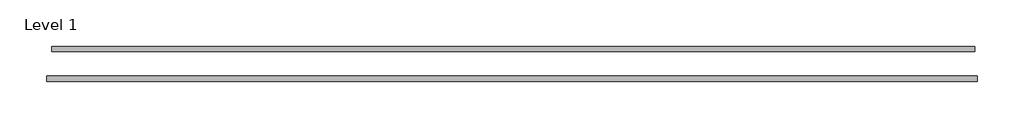
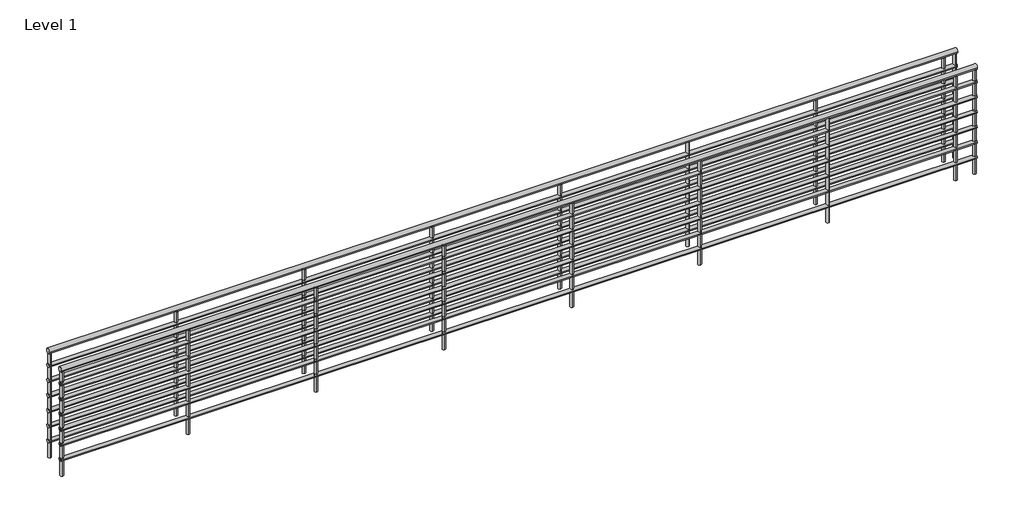
# One storey, part 2 of 2: 2 railings.
"""IFC4 building model written with IfcOpenShell, lengths in millimetres."""

from ifc_helpers import new_model, si_unit, point, frame, frame_2d, origin, origin_with_axes, place, context, project, spatial, circle_curve, trimmed, segment, composite_curve, outline, extrude, element, save

model = new_model("IFC4")

# Units and contexts
model_context = context("Model", 3, world=origin())
ifc_project = project(units=[si_unit("LENGTHUNIT", "METRE", prefix="MILLI")], contexts=[model_context])

# Site, building, storey
site = spatial("IfcSite", under=ifc_project)
building = spatial("IfcBuilding", under=site)
storey = spatial("IfcBuildingStorey", under=building, Name="Level 1", Elevation=0.0)

# Railings
placement = place(None, origin())
element("IfcRailing", 1, ObjectType="900mm Pipe", at=placement, inside=storey, context=model_context, shape_type="SweptSolid", body=[
    extrude(outline(composite_curve([segment(trimmed(circle_curve(frame_2d((34329.0024844, 880.0)), 20.0), [point((34309.0024844, 880.0))], [point((34349.0024844, 880.0))], False, "CARTESIAN"), True, "CONTINUOUS"), segment(trimmed(circle_curve(frame_2d((34329.0024844, 880.0)), 20.0), [point((34349.0024844, 880.0))], [point((34309.0024844, 880.0))], False, "CARTESIAN"), True, "CONTINUOUS")], self_intersect=False)), frame((-2703.3852997, 0.0, 0.0), z_axis=(1.0, 0.0, 0.0), x_axis=(0.0, 1.0, 0.0)), (0.0, 0.0, 1.0), 7100.0),
    extrude(outline(composite_curve([segment(trimmed(circle_curve(frame_2d((34329.0024844, 760.0)), 15.0), [point((34344.0024844, 760.0))], [point((34314.0024844, 760.0))], False, "CARTESIAN"), True, "CONTINUOUS"), segment(trimmed(circle_curve(frame_2d((34329.0024844, 760.0)), 15.0), [point((34314.0024844, 760.0))], [point((34344.0024844, 760.0))], False, "CARTESIAN"), True, "CONTINUOUS")], self_intersect=False)), frame((-2703.3852997, 0.0, 0.0), z_axis=(1.0, 0.0, 0.0), x_axis=(0.0, 1.0, 0.0)), (0.0, 0.0, 1.0), 7100.0),
    extrude(outline(composite_curve([segment(trimmed(circle_curve(frame_2d((34329.0024844, 635.0)), 15.0), [point((34344.0024844, 635.0))], [point((34314.0024844, 635.0))], False, "CARTESIAN"), True, "CONTINUOUS"), segment(trimmed(circle_curve(frame_2d((34329.0024844, 635.0)), 15.0), [point((34314.0024844, 635.0))], [point((34344.0024844, 635.0))], False, "CARTESIAN"), True, "CONTINUOUS")], self_intersect=False)), frame((-2703.3852997, 0.0, 0.0), z_axis=(1.0, 0.0, 0.0), x_axis=(0.0, 1.0, 0.0)), (0.0, 0.0, 1.0), 7100.0),
    extrude(outline(composite_curve([segment(trimmed(circle_curve(frame_2d((34329.0024844, 510.0)), 15.0), [point((34344.0024844, 510.0))], [point((34314.0024844, 510.0))], False, "CARTESIAN"), True, "CONTINUOUS"), segment(trimmed(circle_curve(frame_2d((34329.0024844, 510.0)), 15.0), [point((34314.0024844, 510.0))], [point((34344.0024844, 510.0))], False, "CARTESIAN"), True, "CONTINUOUS")], self_intersect=False)), frame((-2703.3852997, 0.0, 0.0), z_axis=(1.0, 0.0, 0.0), x_axis=(0.0, 1.0, 0.0)), (0.0, 0.0, 1.0), 7100.0),
    extrude(outline(composite_curve([segment(trimmed(circle_curve(frame_2d((34329.0024844, 385.0)), 15.0), [point((34344.0024844, 385.0))], [point((34314.0024844, 385.0))], False, "CARTESIAN"), True, "CONTINUOUS"), segment(trimmed(circle_curve(frame_2d((34329.0024844, 385.0)), 15.0), [point((34314.0024844, 385.0))], [point((34344.0024844, 385.0))], False, "CARTESIAN"), True, "CONTINUOUS")], self_intersect=False)), frame((-2703.3852997, 0.0, 0.0), z_axis=(1.0, 0.0, 0.0), x_axis=(0.0, 1.0, 0.0)), (0.0, 0.0, 1.0), 7100.0),
    extrude(outline(composite_curve([segment(trimmed(circle_curve(frame_2d((34329.0024844, 260.0)), 15.0), [point((34344.0024844, 260.0))], [point((34314.0024844, 260.0))], False, "CARTESIAN"), True, "CONTINUOUS"), segment(trimmed(circle_curve(frame_2d((34329.0024844, 260.0)), 15.0), [point((34314.0024844, 260.0))], [point((34344.0024844, 260.0))], False, "CARTESIAN"), True, "CONTINUOUS")], self_intersect=False)), frame((-2703.3852997, 0.0, 0.0), z_axis=(1.0, 0.0, 0.0), x_axis=(0.0, 1.0, 0.0)), (0.0, 0.0, 1.0), 7100.0),
    extrude(outline(composite_curve([segment(trimmed(circle_curve(frame_2d((34329.0024844, 135.0)), 15.0), [point((34344.0024844, 135.0))], [point((34314.0024844, 135.0))], False, "CARTESIAN"), True, "CONTINUOUS"), segment(trimmed(circle_curve(frame_2d((34329.0024844, 135.0)), 15.0), [point((34314.0024844, 135.0))], [point((34344.0024844, 135.0))], False, "CARTESIAN"), True, "CONTINUOUS")], self_intersect=False)), frame((-2703.3852997, 0.0, 0.0), z_axis=(1.0, 0.0, 0.0), x_axis=(0.0, 1.0, 0.0)), (0.0, 0.0, 1.0), 7100.0),
    extrude(outline(composite_curve([segment(trimmed(circle_curve(frame_2d((4296.6147003, 34329.0024844)), 12.5), [point((4296.6147003, 34341.5024844))], [point((4296.6147003, 34316.5024844))], False, "CARTESIAN"), True, "CONTINUOUS"), segment(trimmed(circle_curve(frame_2d((4296.6147003, 34329.0024844)), 12.5), [point((4296.6147003, 34316.5024844))], [point((4296.6147003, 34341.5024844))], False, "CARTESIAN"), True, "CONTINUOUS")], self_intersect=False)), origin_with_axes(), (0.0, 0.0, 1.0), 860.0),
    extrude(outline(composite_curve([segment(trimmed(circle_curve(frame_2d((3296.6147003, 34329.0024844)), 12.5), [point((3296.6147003, 34341.5024844))], [point((3296.6147003, 34316.5024844))], False, "CARTESIAN"), True, "CONTINUOUS"), segment(trimmed(circle_curve(frame_2d((3296.6147003, 34329.0024844)), 12.5), [point((3296.6147003, 34316.5024844))], [point((3296.6147003, 34341.5024844))], False, "CARTESIAN"), True, "CONTINUOUS")], self_intersect=False)), origin_with_axes(), (0.0, 0.0, 1.0), 860.0),
    extrude(outline(composite_curve([segment(trimmed(circle_curve(frame_2d((2296.6147003, 34329.0024844)), 12.5), [point((2296.6147003, 34341.5024844))], [point((2296.6147003, 34316.5024844))], False, "CARTESIAN"), True, "CONTINUOUS"), segment(trimmed(circle_curve(frame_2d((2296.6147003, 34329.0024844)), 12.5), [point((2296.6147003, 34316.5024844))], [point((2296.6147003, 34341.5024844))], False, "CARTESIAN"), True, "CONTINUOUS")], self_intersect=False)), origin_with_axes(), (0.0, 0.0, 1.0), 860.0),
    extrude(outline(composite_curve([segment(trimmed(circle_curve(frame_2d((1296.6147003, 34329.0024844)), 12.5), [point((1296.6147003, 34341.5024844))], [point((1296.6147003, 34316.5024844))], False, "CARTESIAN"), True, "CONTINUOUS"), segment(trimmed(circle_curve(frame_2d((1296.6147003, 34329.0024844)), 12.5), [point((1296.6147003, 34316.5024844))], [point((1296.6147003, 34341.5024844))], False, "CARTESIAN"), True, "CONTINUOUS")], self_intersect=False)), origin_with_axes(), (0.0, 0.0, 1.0), 860.0),
    extrude(outline(composite_curve([segment(trimmed(circle_curve(frame_2d((296.6147003, 34329.0024844)), 12.5), [point((296.6147003, 34341.5024844))], [point((296.6147003, 34316.5024844))], False, "CARTESIAN"), True, "CONTINUOUS"), segment(trimmed(circle_curve(frame_2d((296.6147003, 34329.0024844)), 12.5), [point((296.6147003, 34316.5024844))], [point((296.6147003, 34341.5024844))], False, "CARTESIAN"), True, "CONTINUOUS")], self_intersect=False)), origin_with_axes(), (0.0, 0.0, 1.0), 860.0),
    extrude(outline(composite_curve([segment(trimmed(circle_curve(frame_2d((-703.3852997, 34329.0024844)), 12.5), [point((-703.3852997, 34341.5024844))], [point((-703.3852997, 34316.5024844))], False, "CARTESIAN"), True, "CONTINUOUS"), segment(trimmed(circle_curve(frame_2d((-703.3852997, 34329.0024844)), 12.5), [point((-703.3852997, 34316.5024844))], [point((-703.3852997, 34341.5024844))], False, "CARTESIAN"), True, "CONTINUOUS")], self_intersect=False)), origin_with_axes(), (0.0, 0.0, 1.0), 860.0),
    extrude(outline(composite_curve([segment(trimmed(circle_curve(frame_2d((-1703.3852997, 34329.0024844)), 12.5), [point((-1703.3852997, 34341.5024844))], [point((-1703.3852997, 34316.5024844))], False, "CARTESIAN"), True, "CONTINUOUS"), segment(trimmed(circle_curve(frame_2d((-1703.3852997, 34329.0024844)), 12.5), [point((-1703.3852997, 34316.5024844))], [point((-1703.3852997, 34341.5024844))], False, "CARTESIAN"), True, "CONTINUOUS")], self_intersect=False)), origin_with_axes(), (0.0, 0.0, 1.0), 860.0),
    extrude(outline(composite_curve([segment(trimmed(circle_curve(frame_2d((4384.1147003, 34329.0024844)), 12.5), [point((4384.1147003, 34341.5024844))], [point((4384.1147003, 34316.5024844))], False, "CARTESIAN"), True, "CONTINUOUS"), segment(trimmed(circle_curve(frame_2d((4384.1147003, 34329.0024844)), 12.5), [point((4384.1147003, 34316.5024844))], [point((4384.1147003, 34341.5024844))], False, "CARTESIAN"), True, "CONTINUOUS")], self_intersect=False)), origin_with_axes(), (0.0, 0.0, 1.0), 860.0),
    extrude(outline(composite_curve([segment(trimmed(circle_curve(frame_2d((-2690.8852997, 34329.0024844)), 12.5), [point((-2690.8852997, 34341.5024844))], [point((-2690.8852997, 34316.5024844))], False, "CARTESIAN"), True, "CONTINUOUS"), segment(trimmed(circle_curve(frame_2d((-2690.8852997, 34329.0024844)), 12.5), [point((-2690.8852997, 34316.5024844))], [point((-2690.8852997, 34341.5024844))], False, "CARTESIAN"), True, "CONTINUOUS")], self_intersect=False)), origin_with_axes(), (0.0, 0.0, 1.0), 860.0),
])
element("IfcRailing", 2, ObjectType="900mm Pipe", at=placement, inside=storey, context=model_context, shape_type="SweptSolid", body=[
    extrude(outline(composite_curve([segment(trimmed(circle_curve(frame_2d((34099.2348375, 880.0)), 20.0), [point((34079.2348375, 880.0))], [point((34119.2348375, 880.0))], False, "CARTESIAN"), True, "CONTINUOUS"), segment(trimmed(circle_curve(frame_2d((34099.2348375, 880.0)), 20.0), [point((34119.2348375, 880.0))], [point((34079.2348375, 880.0))], False, "CARTESIAN"), True, "CONTINUOUS")], self_intersect=False)), frame((-2741.5918674, 0.0, 0.0), z_axis=(1.0, 0.0, 0.0), x_axis=(0.0, 1.0, 0.0)), (0.0, 0.0, 1.0), 7160.0),
    extrude(outline(composite_curve([segment(trimmed(circle_curve(frame_2d((34099.2348375, 760.0)), 15.0), [point((34114.2348375, 760.0))], [point((34084.2348375, 760.0))], False, "CARTESIAN"), True, "CONTINUOUS"), segment(trimmed(circle_curve(frame_2d((34099.2348375, 760.0)), 15.0), [point((34084.2348375, 760.0))], [point((34114.2348375, 760.0))], False, "CARTESIAN"), True, "CONTINUOUS")], self_intersect=False)), frame((-2741.5918674, 0.0, 0.0), z_axis=(1.0, 0.0, 0.0), x_axis=(0.0, 1.0, 0.0)), (0.0, 0.0, 1.0), 7160.0),
    extrude(outline(composite_curve([segment(trimmed(circle_curve(frame_2d((34099.2348375, 635.0)), 15.0), [point((34114.2348375, 635.0))], [point((34084.2348375, 635.0))], False, "CARTESIAN"), True, "CONTINUOUS"), segment(trimmed(circle_curve(frame_2d((34099.2348375, 635.0)), 15.0), [point((34084.2348375, 635.0))], [point((34114.2348375, 635.0))], False, "CARTESIAN"), True, "CONTINUOUS")], self_intersect=False)), frame((-2741.5918674, 0.0, 0.0), z_axis=(1.0, 0.0, 0.0), x_axis=(0.0, 1.0, 0.0)), (0.0, 0.0, 1.0), 7160.0),
    extrude(outline(composite_curve([segment(trimmed(circle_curve(frame_2d((34099.2348375, 510.0)), 15.0), [point((34114.2348375, 510.0))], [point((34084.2348375, 510.0))], False, "CARTESIAN"), True, "CONTINUOUS"), segment(trimmed(circle_curve(frame_2d((34099.2348375, 510.0)), 15.0), [point((34084.2348375, 510.0))], [point((34114.2348375, 510.0))], False, "CARTESIAN"), True, "CONTINUOUS")], self_intersect=False)), frame((-2741.5918674, 0.0, 0.0), z_axis=(1.0, 0.0, 0.0), x_axis=(0.0, 1.0, 0.0)), (0.0, 0.0, 1.0), 7160.0),
    extrude(outline(composite_curve([segment(trimmed(circle_curve(frame_2d((34099.2348375, 385.0)), 15.0), [point((34114.2348375, 385.0))], [point((34084.2348375, 385.0))], False, "CARTESIAN"), True, "CONTINUOUS"), segment(trimmed(circle_curve(frame_2d((34099.2348375, 385.0)), 15.0), [point((34084.2348375, 385.0))], [point((34114.2348375, 385.0))], False, "CARTESIAN"), True, "CONTINUOUS")], self_intersect=False)), frame((-2741.5918674, 0.0, 0.0), z_axis=(1.0, 0.0, 0.0), x_axis=(0.0, 1.0, 0.0)), (0.0, 0.0, 1.0), 7160.0),
    extrude(outline(composite_curve([segment(trimmed(circle_curve(frame_2d((34099.2348375, 260.0)), 15.0), [point((34114.2348375, 260.0))], [point((34084.2348375, 260.0))], False, "CARTESIAN"), True, "CONTINUOUS"), segment(trimmed(circle_curve(frame_2d((34099.2348375, 260.0)), 15.0), [point((34084.2348375, 260.0))], [point((34114.2348375, 260.0))], False, "CARTESIAN"), True, "CONTINUOUS")], self_intersect=False)), frame((-2741.5918674, 0.0, 0.0), z_axis=(1.0, 0.0, 0.0), x_axis=(0.0, 1.0, 0.0)), (0.0, 0.0, 1.0), 7160.0),
    extrude(outline(composite_curve([segment(trimmed(circle_curve(frame_2d((34099.2348375, 135.0)), 15.0), [point((34114.2348375, 135.0))], [point((34084.2348375, 135.0))], False, "CARTESIAN"), True, "CONTINUOUS"), segment(trimmed(circle_curve(frame_2d((34099.2348375, 135.0)), 15.0), [point((34084.2348375, 135.0))], [point((34114.2348375, 135.0))], False, "CARTESIAN"), True, "CONTINUOUS")], self_intersect=False)), frame((-2741.5918674, 0.0, 0.0), z_axis=(1.0, 0.0, 0.0), x_axis=(0.0, 1.0, 0.0)), (0.0, 0.0, 1.0), 7160.0),
    extrude(outline(composite_curve([segment(trimmed(circle_curve(frame_2d((4258.4081326, 34099.2348375)), 12.5), [point((4258.4081326, 34111.7348375))], [point((4258.4081326, 34086.7348375))], False, "CARTESIAN"), True, "CONTINUOUS"), segment(trimmed(circle_curve(frame_2d((4258.4081326, 34099.2348375)), 12.5), [point((4258.4081326, 34086.7348375))], [point((4258.4081326, 34111.7348375))], False, "CARTESIAN"), True, "CONTINUOUS")], self_intersect=False)), origin_with_axes(), (0.0, 0.0, 1.0), 860.0),
    extrude(outline(composite_curve([segment(trimmed(circle_curve(frame_2d((3258.4081326, 34099.2348375)), 12.5), [point((3258.4081326, 34111.7348375))], [point((3258.4081326, 34086.7348375))], False, "CARTESIAN"), True, "CONTINUOUS"), segment(trimmed(circle_curve(frame_2d((3258.4081326, 34099.2348375)), 12.5), [point((3258.4081326, 34086.7348375))], [point((3258.4081326, 34111.7348375))], False, "CARTESIAN"), True, "CONTINUOUS")], self_intersect=False)), origin_with_axes(), (0.0, 0.0, 1.0), 860.0),
    extrude(outline(composite_curve([segment(trimmed(circle_curve(frame_2d((2258.4081326, 34099.2348375)), 12.5), [point((2258.4081326, 34111.7348375))], [point((2258.4081326, 34086.7348375))], False, "CARTESIAN"), True, "CONTINUOUS"), segment(trimmed(circle_curve(frame_2d((2258.4081326, 34099.2348375)), 12.5), [point((2258.4081326, 34086.7348375))], [point((2258.4081326, 34111.7348375))], False, "CARTESIAN"), True, "CONTINUOUS")], self_intersect=False)), origin_with_axes(), (0.0, 0.0, 1.0), 860.0),
    extrude(outline(composite_curve([segment(trimmed(circle_curve(frame_2d((1258.4081326, 34099.2348375)), 12.5), [point((1258.4081326, 34111.7348375))], [point((1258.4081326, 34086.7348375))], False, "CARTESIAN"), True, "CONTINUOUS"), segment(trimmed(circle_curve(frame_2d((1258.4081326, 34099.2348375)), 12.5), [point((1258.4081326, 34086.7348375))], [point((1258.4081326, 34111.7348375))], False, "CARTESIAN"), True, "CONTINUOUS")], self_intersect=False)), origin_with_axes(), (0.0, 0.0, 1.0), 860.0),
    extrude(outline(composite_curve([segment(trimmed(circle_curve(frame_2d((258.4081326, 34099.2348375)), 12.5), [point((258.4081326, 34111.7348375))], [point((258.4081326, 34086.7348375))], False, "CARTESIAN"), True, "CONTINUOUS"), segment(trimmed(circle_curve(frame_2d((258.4081326, 34099.2348375)), 12.5), [point((258.4081326, 34086.7348375))], [point((258.4081326, 34111.7348375))], False, "CARTESIAN"), True, "CONTINUOUS")], self_intersect=False)), origin_with_axes(), (0.0, 0.0, 1.0), 860.0),
    extrude(outline(composite_curve([segment(trimmed(circle_curve(frame_2d((-741.5918674, 34099.2348375)), 12.5), [point((-741.5918674, 34111.7348375))], [point((-741.5918674, 34086.7348375))], False, "CARTESIAN"), True, "CONTINUOUS"), segment(trimmed(circle_curve(frame_2d((-741.5918674, 34099.2348375)), 12.5), [point((-741.5918674, 34086.7348375))], [point((-741.5918674, 34111.7348375))], False, "CARTESIAN"), True, "CONTINUOUS")], self_intersect=False)), origin_with_axes(), (0.0, 0.0, 1.0), 860.0),
    extrude(outline(composite_curve([segment(trimmed(circle_curve(frame_2d((-1741.5918674, 34099.2348375)), 12.5), [point((-1741.5918674, 34111.7348375))], [point((-1741.5918674, 34086.7348375))], False, "CARTESIAN"), True, "CONTINUOUS"), segment(trimmed(circle_curve(frame_2d((-1741.5918674, 34099.2348375)), 12.5), [point((-1741.5918674, 34086.7348375))], [point((-1741.5918674, 34111.7348375))], False, "CARTESIAN"), True, "CONTINUOUS")], self_intersect=False)), origin_with_axes(), (0.0, 0.0, 1.0), 860.0),
    extrude(outline(composite_curve([segment(trimmed(circle_curve(frame_2d((4405.9081326, 34099.2348375)), 12.5), [point((4405.9081326, 34111.7348375))], [point((4405.9081326, 34086.7348375))], False, "CARTESIAN"), True, "CONTINUOUS"), segment(trimmed(circle_curve(frame_2d((4405.9081326, 34099.2348375)), 12.5), [point((4405.9081326, 34086.7348375))], [point((4405.9081326, 34111.7348375))], False, "CARTESIAN"), True, "CONTINUOUS")], self_intersect=False)), origin_with_axes(), (0.0, 0.0, 1.0), 860.0),
    extrude(outline(composite_curve([segment(trimmed(circle_curve(frame_2d((-2729.0918674, 34099.2348375)), 12.5), [point((-2729.0918674, 34111.7348375))], [point((-2729.0918674, 34086.7348375))], False, "CARTESIAN"), True, "CONTINUOUS"), segment(trimmed(circle_curve(frame_2d((-2729.0918674, 34099.2348375)), 12.5), [point((-2729.0918674, 34086.7348375))], [point((-2729.0918674, 34111.7348375))], False, "CARTESIAN"), True, "CONTINUOUS")], self_intersect=False)), origin_with_axes(), (0.0, 0.0, 1.0), 860.0),
])

save(model, "model.ifc")

# Revit data of these elements
# Type "900mm Pipe"
#   built-in parameter 1008612 = 0.019685 (stored number, unit not read)
#   built-in parameter 1008611 = 0.0984252 (stored number, unit not read)
#   built-in parameter 1008609 = 6.56168 (stored number, unit not read)
#   built-in parameter 1008604 = 0.19685 (stored number, unit not read)
#   built-in parameter 1008603 = 0.164042 (stored number, unit not read)
#   Railing Height = 2' - 11.43307"
#   built-in parameter 1008630 = 2
#   built-in parameter 1008610 = 2
#   built-in parameter 1008605 = 1
#   built-in parameter 1008618 = M_Baluster - Round : 25mm
# Elements 1, 2 (IfcRailing, "900mm Pipe")
#   Phase Created = New Construction
